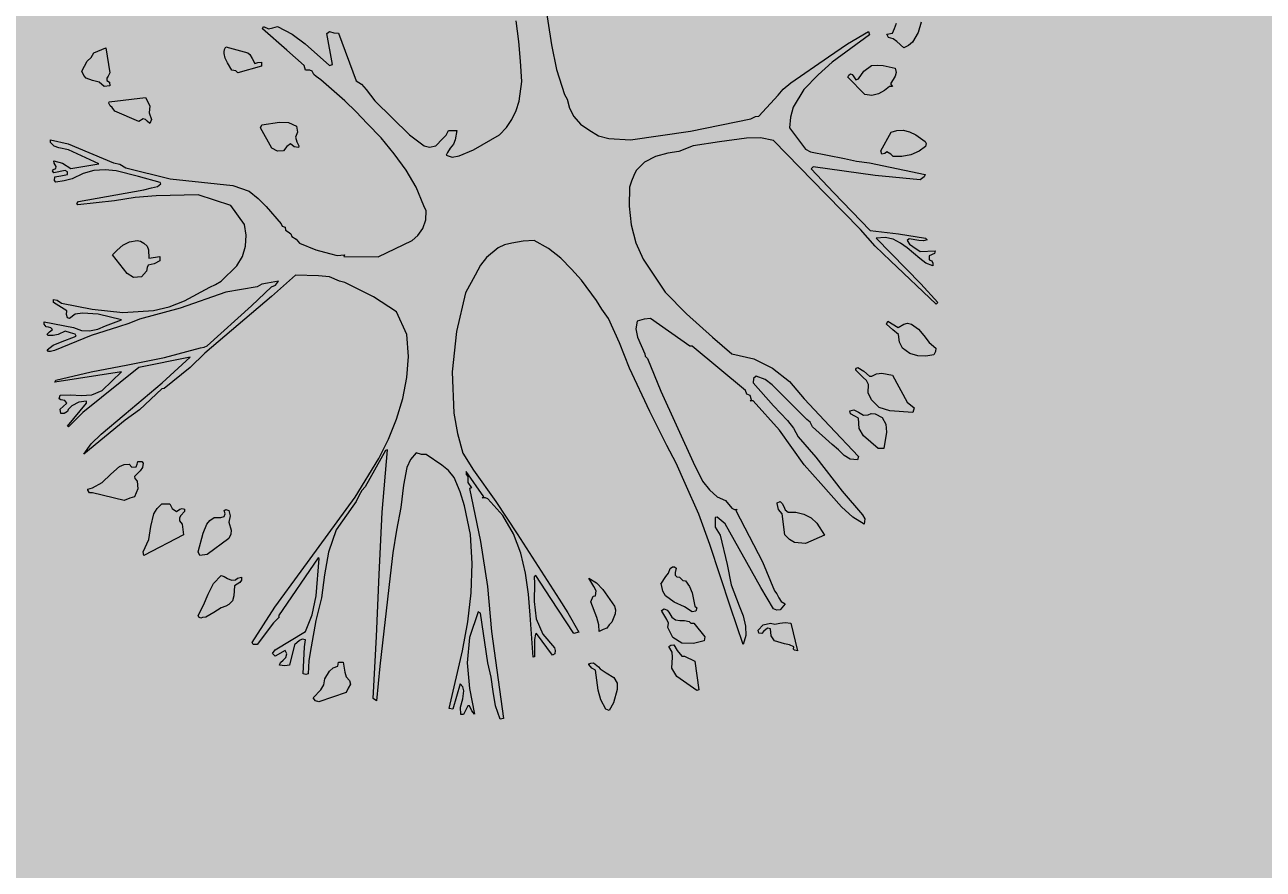
# Model space of a CAD drawing. Units: inches. Extents: x 84 to 1044, y -280 to 906.
# Tile 92 of 105: x 749 to 779, y 479 to 499. Entities that reach past the tile are written whole.
import ezdxf

# ---------------------------------------------------------------- set-up
doc = ezdxf.new("R2010")
doc.units = ezdxf.units.IN
doc.layers.add('A-ANNO-DIMS', color=2, linetype='Continuous', lineweight=18)
doc.layers.add('L-PLNT', color=114, linetype='Continuous', lineweight=15)
doc.layers.add('L-PLNT-PATT', color=9, linetype='Continuous', lineweight=9, true_color=0xafd9aa)
doc.styles.get("Standard").update_dxf_attribs({"font": 'arial.ttf'})
doc.dimstyles.get("Standard").update_dxf_attribs({"dimtxt": 0.18, "dimasz": 0.18, "dimexe": 0.18, "dimexo": 0.0625, "dimgap": 0.09, "dimtad": 0, "dimtih": 1, "dimtoh": 1, "dimdec": 4, "dimzin": 0, "dimdsep": 46, "dimtxsty": 'Standard', "dimcen": 0.09, "dimadec": 0, "dimazin": 0, "dimtfac": 1, "dimtdec": 4, "dimtofl": 0, "dimtmove": 0, "dimatfit": 3, "dimfxl": 1, "dimtolj": 1, "dimtzin": 0, "dimarcsym": 0})

# ---------------------------------------------------------------- blocks, each defined once
blk = doc.blocks.new('A$C37E508DF')
for p, q in [((0.7911, 1.1436), (0.8027, 1.0677)), ((0.7512, 1.0728), (0.7469, 1.1054)), ((1.3455, 1.0934), (1.3485, 1.102)), ((1.3875, 1.1037), (1.3828, 1.087)), ((0.3456, 1.093), (0.3469, 1.0964)), ((0.3842, 1.0591), (0.3456, 1.093)), ((0.3469, 1.0964), (0.355, 1.093)), ((0.355, 1.093), (0.3619, 1.0943)), ((0.3619, 1.0943), (0.3692, 1.0968)), ((0.3692, 1.0968), (0.3923, 1.0844)), ((0.3923, 1.0844), (0.4129, 1.069)), ((0.4472, 1.0857), (0.4515, 1.0887)), ((0.4562, 1.0364), (0.4472, 1.0857)), ((0.4515, 1.0887), (0.4584, 1.0865)), ((0.4584, 1.0865), (0.4657, 1.0861)), ((0.4657, 1.0861), (0.4939, 1.0107)), ((1.3057, 1.0835), (1.2469, 1.0402)), ((1.2713, 1.0694), (1.3044, 1.0887)), ((1.3044, 1.0887), (1.3057, 1.0835)), ((1.3335, 1.0844), (1.3421, 1.0861)), ((1.3361, 1.0793), (1.3335, 1.0844)), ((1.3434, 1.0771), (1.3361, 1.0793)), ((1.3421, 1.0861), (1.3455, 1.0934)), ((1.3828, 1.087), (1.3738, 1.072)), ((0.0789, 1.0552), (0.0978, 1.063)), ((0.0978, 1.063), (0.1042, 1.0231)), ((0.2847, 1.0565), (0.2856, 1.0604)), ((0.2856, 1.0604), (0.2877, 1.0647)), ((0.2877, 1.0647), (0.3224, 1.0552)), ((0.4112, 1.0351), (0.3842, 1.0591)), ((0.4129, 1.069), (0.4515, 1.0351)), ((0.7538, 1.0415), (0.7512, 1.0728)), ((0.8027, 1.0677), (0.8108, 1.0287)), ((1.2409, 1.0488), (1.2713, 1.0694)), ((1.349, 1.0728), (1.3434, 1.0771)), ((1.3605, 1.063), (1.349, 1.0728)), ((1.3678, 1.0664), (1.3605, 1.063)), ((1.3738, 1.072), (1.3678, 1.0664)), ((0.0596, 1.0257), (0.0682, 1.0415)), ((0.0682, 1.0415), (0.0746, 1.0475)), ((0.0746, 1.0475), (0.0789, 1.0552)), ((0.2851, 1.054), (0.2847, 1.0565)), ((0.2864, 1.0463), (0.2851, 1.054)), ((0.2899, 1.039), (0.2864, 1.0463)), ((0.2972, 1.0274), (0.2899, 1.039)), ((0.3224, 1.0552), (0.3255, 1.0522)), ((0.3255, 1.0522), (0.3293, 1.0458)), ((0.3293, 1.0458), (0.3336, 1.0381)), ((0.3336, 1.0381), (0.3383, 1.0398)), ((0.3383, 1.0398), (0.3439, 1.0402)), ((0.3439, 1.0402), (0.3439, 1.0338)), ((0.7559, 1.0098), (0.7538, 1.0415)), ((1.1813, 1.0072), (1.2409, 1.0488)), ((1.2469, 1.0402), (1.2246, 1.0201)), ((0.0626, 1.0188), (0.0596, 1.0257)), ((0.1042, 1.0231), (0.1012, 1.018)), ((0.3032, 1.0265), (0.2972, 1.0274)), ((0.3066, 1.0231), (0.3032, 1.0265)), ((0.3439, 1.0338), (0.3066, 1.0231)), ((0.4138, 1.0274), (0.4112, 1.0351)), ((0.4202, 1.0274), (0.4138, 1.0274)), ((0.4241, 1.0257), (0.4202, 1.0274)), ((0.4267, 1.0209), (0.4241, 1.0257)), ((0.4305, 1.0175), (0.4267, 1.0209)), ((0.4515, 1.0351), (0.4562, 1.0364)), ((0.8108, 1.0287), (0.8233, 0.9892)), ((1.2246, 1.0201), (1.2023, 0.9969)), ((1.2718, 1.0162), (1.2731, 1.0197)), ((1.2731, 1.0197), (1.2761, 1.0218)), ((1.2761, 1.0218), (1.2786, 1.0209)), ((1.2786, 1.0209), (1.2799, 1.0184)), ((1.2885, 1.0136), (1.2971, 1.0257)), ((1.2971, 1.0257), (1.3091, 1.0351)), ((1.3091, 1.0351), (1.3185, 1.0355)), ((1.3185, 1.0355), (1.3275, 1.0347)), ((1.3275, 1.0347), (1.3468, 1.0308)), ((1.3468, 1.0308), (1.3481, 1.0239)), ((1.3481, 1.0239), (1.3468, 1.018)), ((0.0665, 1.0149), (0.0626, 1.0188)), ((0.0763, 1.0111), (0.0665, 1.0149)), ((0.087, 1.0085), (0.0763, 1.0111)), ((0.0948, 1.0016), (0.087, 1.0085)), ((0.1042, 1.0029), (0.0948, 1.0016)), ((0.1012, 1.018), (0.099, 1.0149)), ((0.099, 1.0149), (0.099, 1.0111)), ((0.099, 1.0111), (0.1033, 1.0085)), ((0.1033, 1.0085), (0.1042, 1.0029)), ((0.4378, 1.0124), (0.4305, 1.0175)), ((0.476, 0.9789), (0.4378, 1.0124)), ((0.4939, 1.0107), (0.5021, 1.0051)), ((0.5021, 1.0051), (0.5094, 0.9969)), ((0.7516, 0.9785), (0.7559, 1.0098)), ((1.1693, 0.9974), (1.1813, 1.0072)), ((1.2984, 0.9892), (1.2718, 1.0162)), ((1.2799, 1.0184), (1.2842, 1.0124)), ((1.2842, 1.0124), (1.2885, 1.0136)), ((1.3378, 1.0016), (1.3297, 0.9952)), ((1.3421, 1.0016), (1.3378, 1.0016)), ((1.3468, 1.018), (1.3391, 1.0059)), ((1.3391, 1.0059), (1.3421, 1.0016)), ((0.1029, 0.9772), (0.1604, 0.9841)), ((0.1604, 0.9841), (0.1672, 0.9708)), ((0.5094, 0.9969), (0.5231, 0.9789)), ((0.8233, 0.9892), (0.8275, 0.9815)), ((0.8275, 0.9815), (0.8314, 0.9673)), ((1.1311, 0.9549), (1.1612, 0.9879)), ((1.1612, 0.9879), (1.1693, 0.9974)), ((1.2023, 0.9969), (1.1852, 0.9691)), ((1.3095, 0.9875), (1.2984, 0.9892)), ((1.3202, 0.9901), (1.3095, 0.9875)), ((1.3297, 0.9952), (1.3202, 0.9901)), ((0.1025, 0.9751), (0.1029, 0.9772)), ((0.1046, 0.9708), (0.1025, 0.9751)), ((0.1076, 0.9682), (0.1046, 0.9708)), ((0.1119, 0.9626), (0.1076, 0.9682)), ((0.1496, 0.9463), (0.1119, 0.9626)), ((0.1672, 0.9708), (0.1664, 0.9601)), ((0.4939, 0.9618), (0.476, 0.9789)), ((0.5111, 0.9429), (0.4939, 0.9618)), ((0.5231, 0.9789), (0.578, 0.9253)), ((0.7401, 0.9493), (0.7469, 0.9635)), ((0.7469, 0.9635), (0.7516, 0.9785)), ((0.8314, 0.9673), (0.8383, 0.954)), ((1.1852, 0.9691), (1.1809, 0.9532)), ((0.1565, 0.9506), (0.1496, 0.9463)), ((0.1604, 0.9493), (0.1565, 0.9506)), ((0.1629, 0.9468), (0.1604, 0.9493)), ((0.1672, 0.9429), (0.1629, 0.9468)), ((0.1664, 0.9601), (0.1698, 0.9493)), ((0.1698, 0.9493), (0.1672, 0.9429)), ((0.3426, 0.936), (0.3443, 0.9412)), ((0.3443, 0.9412), (0.3722, 0.9451)), ((0.3722, 0.9451), (0.3868, 0.9446)), ((0.3868, 0.9446), (0.3992, 0.9386)), ((0.5334, 0.9202), (0.5111, 0.9429)), ((0.7315, 0.9365), (0.7401, 0.9493)), ((0.8383, 0.954), (0.8486, 0.942)), ((0.8486, 0.942), (0.8619, 0.933)), ((1.0227, 0.9309), (1.1183, 0.9506)), ((1.1183, 0.9506), (1.1256, 0.954)), ((1.1256, 0.954), (1.1311, 0.9549)), ((1.1809, 0.9532), (1.1796, 0.936)), ((0.3602, 0.9039), (0.3426, 0.936)), ((0.4009, 0.9292), (0.3975, 0.9215)), ((0.3975, 0.9215), (0.3996, 0.9142)), ((0.3992, 0.9386), (0.4009, 0.9292)), ((0.578, 0.9253), (0.6011, 0.9077)), ((0.6303, 0.9189), (0.6359, 0.9245)), ((0.6359, 0.9245), (0.6397, 0.9322)), ((0.6397, 0.9322), (0.653, 0.9322)), ((0.653, 0.9322), (0.6505, 0.9172)), ((0.6796, 0.9013), (0.7203, 0.9253)), ((0.7203, 0.9253), (0.7315, 0.9365)), ((0.8619, 0.933), (0.8769, 0.9236)), ((0.8769, 0.9236), (0.8936, 0.9193)), ((0.9279, 0.9172), (1.0227, 0.9309)), ((1.1796, 0.936), (1.2049, 0.9022)), ((1.3241, 0.9), (1.3404, 0.9292)), ((1.3404, 0.9292), (1.3494, 0.9322)), ((1.3494, 0.9322), (1.3592, 0.9326)), ((1.3592, 0.9326), (1.3695, 0.93)), ((1.3695, 0.93), (1.3794, 0.9253)), ((1.3794, 0.9253), (1.394, 0.9146)), ((0.0103, 0.9129), (0.0103, 0.9172)), ((0.0103, 0.9172), (0.0382, 0.9107)), ((0.0159, 0.9073), (0.0103, 0.9129)), ((0.0232, 0.9043), (0.0159, 0.9073)), ((0.0386, 0.9013), (0.0232, 0.9043)), ((0.0382, 0.9107), (0.1098, 0.8807)), ((0.3692, 0.8992), (0.3602, 0.9039)), ((0.3838, 0.9069), (0.379, 0.9)), ((0.3898, 0.9107), (0.3838, 0.9069)), ((0.3958, 0.906), (0.3898, 0.9107)), ((0.4026, 0.9052), (0.3958, 0.906)), ((0.3996, 0.9142), (0.4031, 0.9077)), ((0.4031, 0.9077), (0.4026, 0.9052)), ((0.554, 0.8953), (0.5334, 0.9202)), ((0.6011, 0.9077), (0.6097, 0.9056)), ((0.6097, 0.9056), (0.6196, 0.9077)), ((0.6196, 0.9077), (0.6303, 0.9189)), ((0.6423, 0.9039), (0.6384, 0.8974)), ((0.6479, 0.9103), (0.6423, 0.9039)), ((0.6505, 0.9172), (0.6479, 0.9103)), ((0.8936, 0.9193), (0.9279, 0.9172)), ((1.0269, 0.9077), (1.0042, 0.8987)), ((1.0685, 0.9142), (1.0269, 0.9077)), ((1.1114, 0.9198), (1.0685, 0.9142)), ((1.1333, 0.9202), (1.1114, 0.9198)), ((1.1543, 0.9159), (1.1333, 0.9202)), ((1.2371, 0.8314), (1.1543, 0.9159)), ((1.2049, 0.9022), (1.2126, 0.8983)), ((1.3948, 0.9065), (1.3846, 0.8992)), ((1.394, 0.9146), (1.3957, 0.9112)), ((1.3957, 0.9112), (1.3948, 0.9065)), ((0.0159, 0.8803), (0.0154, 0.8837)), ((0.0154, 0.8837), (0.0292, 0.8803)), ((0.0866, 0.8794), (0.0386, 0.9013)), ((0.379, 0.9), (0.3692, 0.8992)), ((0.5728, 0.8691), (0.554, 0.8953)), ((0.6384, 0.8974), (0.6359, 0.8927)), ((0.6359, 0.8927), (0.6457, 0.8897)), ((0.6457, 0.8897), (0.6569, 0.8919)), ((0.6569, 0.8919), (0.6796, 0.9013)), ((0.9673, 0.8906), (0.9498, 0.8816)), ((0.9866, 0.8962), (0.9673, 0.8906)), ((1.0042, 0.8987), (0.9866, 0.8962)), ((1.2126, 0.8983), (1.2662, 0.8876)), ((1.2662, 0.8876), (1.2855, 0.8833)), ((1.2855, 0.8833), (1.3057, 0.8807)), ((1.3254, 0.8944), (1.3241, 0.9)), ((1.3301, 0.8957), (1.3254, 0.8944)), ((1.3335, 0.8983), (1.3301, 0.8957)), ((1.3395, 0.8944), (1.3335, 0.8983)), ((1.3434, 0.8906), (1.3395, 0.8944)), ((1.3571, 0.8906), (1.3434, 0.8906)), ((1.3713, 0.8936), (1.3571, 0.8906)), ((1.3846, 0.8992), (1.3713, 0.8936)), ((0.0133, 0.8679), (0.015, 0.87)), ((0.0154, 0.8649), (0.0133, 0.8679)), ((0.015, 0.87), (0.0184, 0.8717)), ((0.0334, 0.8687), (0.0154, 0.8649)), ((0.0176, 0.8777), (0.0159, 0.8803)), ((0.0193, 0.8752), (0.0176, 0.8777)), ((0.0184, 0.8717), (0.0193, 0.8752)), ((0.0266, 0.8602), (0.0369, 0.8623)), ((0.0292, 0.8803), (0.0424, 0.8717)), ((0.0369, 0.8666), (0.0334, 0.8687)), ((0.0369, 0.8623), (0.0369, 0.8666)), ((0.0424, 0.8717), (0.0866, 0.8794)), ((0.0617, 0.864), (0.0442, 0.8554)), ((0.0789, 0.8687), (0.0617, 0.864)), ((0.0965, 0.8696), (0.0789, 0.8687)), ((0.1141, 0.8679), (0.0965, 0.8696)), ((0.1098, 0.8807), (0.1196, 0.8786)), ((0.1492, 0.8593), (0.1141, 0.8679)), ((0.1196, 0.8786), (0.1295, 0.873)), ((0.1295, 0.873), (0.1994, 0.8554)), ((0.5887, 0.8421), (0.5728, 0.8691)), ((0.9369, 0.8687), (0.933, 0.861)), ((0.9498, 0.8816), (0.9369, 0.8687)), ((1.2169, 0.8743), (1.2135, 0.8713)), ((1.2135, 0.8713), (1.2491, 0.834)), ((1.3151, 0.8606), (1.2169, 0.8743)), ((1.3057, 0.8807), (1.394, 0.8623)), ((1.394, 0.8623), (1.3927, 0.8584)), ((0.0163, 0.8529), (0.0171, 0.8584)), ((0.0184, 0.8503), (0.0163, 0.8529)), ((0.0171, 0.8584), (0.0266, 0.8602)), ((0.0317, 0.8524), (0.0184, 0.8503)), ((0.0442, 0.8554), (0.0317, 0.8524)), ((0.1835, 0.8499), (0.1492, 0.8593)), ((0.1698, 0.8413), (0.1792, 0.8434)), ((0.1792, 0.8434), (0.1848, 0.8477)), ((0.1848, 0.8477), (0.1835, 0.8499)), ((0.1994, 0.8554), (0.2984, 0.8447)), ((0.2984, 0.8447), (0.3242, 0.8357)), ((0.9296, 0.852), (0.9262, 0.8421)), ((0.933, 0.861), (0.9296, 0.852)), ((1.3863, 0.8541), (1.3151, 0.8606)), ((1.3927, 0.8584), (1.3863, 0.8541)), ((0.0545, 0.8194), (0.1578, 0.8378)), ((0.1441, 0.8258), (0.1111, 0.8207)), ((0.1771, 0.8288), (0.1441, 0.8258)), ((0.1578, 0.8378), (0.1698, 0.8413)), ((0.2436, 0.8301), (0.1771, 0.8288)), ((0.2954, 0.813), (0.2436, 0.8301)), ((0.3242, 0.8357), (0.3387, 0.8241)), ((0.3387, 0.8241), (0.3512, 0.8117)), ((0.6007, 0.8125), (0.5887, 0.8421)), ((0.9262, 0.8421), (0.9257, 0.8121)), ((1.2919, 0.7752), (1.2371, 0.8314)), ((1.2491, 0.834), (1.3069, 0.7735)), ((0.0519, 0.8164), (0.0545, 0.8194)), ((0.0532, 0.8143), (0.0519, 0.8164)), ((0.1111, 0.8207), (0.0532, 0.8143)), ((0.3173, 0.7834), (0.2954, 0.813)), ((0.3512, 0.8117), (0.3748, 0.7842)), ((0.6046, 0.8048), (0.6007, 0.8125)), ((0.6037, 0.7903), (0.6046, 0.8048)), ((0.9257, 0.8121), (0.9287, 0.7825)), ((0.3748, 0.7842), (0.3765, 0.7804)), ((0.599, 0.777), (0.6037, 0.7903)), ((0.3199, 0.7662), (0.3173, 0.7834)), ((0.3186, 0.7491), (0.3199, 0.7662)), ((0.3765, 0.7804), (0.3816, 0.7791)), ((0.3816, 0.7791), (0.382, 0.7744)), ((0.382, 0.7744), (0.3859, 0.7714)), ((0.3859, 0.7714), (0.3902, 0.7684)), ((0.3902, 0.7684), (0.3919, 0.7641)), ((0.5823, 0.7577), (0.5913, 0.7658)), ((0.5913, 0.7658), (0.599, 0.777)), ((0.9287, 0.7825), (0.936, 0.7542)), ((1.3151, 0.7487), (1.2919, 0.7752)), ((1.3069, 0.7735), (1.352, 0.7684)), ((1.352, 0.7684), (1.3948, 0.7615)), ((0.1153, 0.7427), (0.1244, 0.7504)), ((0.1244, 0.7504), (0.1351, 0.7559)), ((0.1351, 0.7559), (0.1471, 0.7577)), ((0.1471, 0.7577), (0.1527, 0.7568)), ((0.1527, 0.7568), (0.1578, 0.7538)), ((0.1578, 0.7538), (0.1629, 0.7491)), ((0.1629, 0.7491), (0.1651, 0.7431)), ((0.3139, 0.7324), (0.3186, 0.7491)), ((0.3919, 0.7641), (0.3988, 0.7598)), ((0.3988, 0.7598), (0.4043, 0.7538)), ((0.4043, 0.7538), (0.4301, 0.7431)), ((0.5287, 0.7319), (0.5823, 0.7577)), ((0.7182, 0.7461), (0.7002, 0.7307)), ((0.7285, 0.7512), (0.7182, 0.7461)), ((0.7401, 0.7534), (0.7285, 0.7512)), ((0.7577, 0.7568), (0.7401, 0.7534)), ((0.7752, 0.7577), (0.7577, 0.7568)), ((0.798, 0.7452), (0.7752, 0.7577)), ((0.8173, 0.7298), (0.798, 0.7452)), ((0.936, 0.7542), (0.9476, 0.7285)), ((1.3391, 0.7255), (1.3151, 0.7487)), ((1.3309, 0.7624), (1.3164, 0.7615)), ((1.3164, 0.7615), (1.3871, 0.6891)), ((1.3434, 0.7598), (1.3309, 0.7624)), ((1.355, 0.7538), (1.3434, 0.7598)), ((1.3653, 0.7461), (1.355, 0.7538)), ((1.3854, 0.7294), (1.3653, 0.7461)), ((1.3687, 0.7607), (1.3657, 0.7577)), ((1.3657, 0.7577), (1.3691, 0.7521)), ((1.3841, 0.7577), (1.3687, 0.7607)), ((1.3691, 0.7521), (1.3743, 0.7482)), ((1.3743, 0.7482), (1.3863, 0.7405)), ((1.3914, 0.7572), (1.3841, 0.7577)), ((1.397, 0.759), (1.3914, 0.7572)), ((1.3948, 0.7615), (1.397, 0.759)), ((0.1081, 0.7349), (0.1153, 0.7427)), ((0.1312, 0.7058), (0.1081, 0.7349)), ((0.1651, 0.7431), (0.1655, 0.7298)), ((0.1655, 0.7298), (0.1831, 0.7324)), ((0.1831, 0.7255), (0.1741, 0.7208)), ((0.1831, 0.7324), (0.1831, 0.7255)), ((0.3049, 0.7178), (0.3139, 0.7324)), ((0.4301, 0.7431), (0.4515, 0.7371)), ((0.4515, 0.7371), (0.4635, 0.7341)), ((0.4635, 0.7341), (0.4755, 0.7349)), ((0.4755, 0.7349), (0.4742, 0.7324)), ((0.4742, 0.7324), (0.5287, 0.7319)), ((0.7002, 0.7307), (0.6903, 0.7186)), ((0.8344, 0.7122), (0.8173, 0.7298)), ((0.9476, 0.7285), (0.9828, 0.6762)), ((1.4116, 0.6569), (1.3391, 0.7255)), ((1.3953, 0.7221), (1.3854, 0.7294)), ((1.3863, 0.7405), (1.4099, 0.7414)), ((1.4086, 0.7375), (1.4004, 0.7337)), ((1.4004, 0.7337), (1.4004, 0.7272)), ((1.4004, 0.7272), (1.4047, 0.7255)), ((1.4047, 0.7255), (1.406, 0.7221)), ((1.4099, 0.7414), (1.4086, 0.7375)), ((0.1415, 0.6994), (0.1312, 0.7058)), ((0.1621, 0.7092), (0.1539, 0.7002)), ((0.1629, 0.7152), (0.1621, 0.7092)), ((0.1646, 0.7186), (0.1629, 0.7152)), ((0.1741, 0.7208), (0.1646, 0.7186)), ((0.28, 0.6933), (0.3049, 0.7178)), ((0.6903, 0.7186), (0.6818, 0.7032)), ((0.8503, 0.6951), (0.8344, 0.7122)), ((1.4064, 0.7178), (1.3953, 0.7221)), ((1.406, 0.7221), (1.4064, 0.7178)), ((0.1539, 0.7002), (0.1415, 0.6994)), ((0.262, 0.6839), (0.271, 0.6882)), ((0.271, 0.6882), (0.28, 0.6933)), ((0.3443, 0.6886), (0.337, 0.6843)), ((0.3533, 0.6903), (0.3443, 0.6886)), ((0.3709, 0.6933), (0.3533, 0.6903)), ((0.3975, 0.7028), (0.3598, 0.6693)), ((0.3598, 0.6843), (0.3662, 0.6873)), ((0.3662, 0.6873), (0.3709, 0.6933)), ((0.4339, 0.7019), (0.3975, 0.7028)), ((0.4515, 0.7002), (0.4339, 0.7019)), ((0.4674, 0.6933), (0.4515, 0.7002)), ((0.476, 0.6912), (0.4674, 0.6933)), ((0.4832, 0.6878), (0.476, 0.6912)), ((0.521, 0.6685), (0.4832, 0.6878)), ((0.6818, 0.7032), (0.6667, 0.6749)), ((0.8739, 0.6629), (0.8503, 0.6951)), ((1.3871, 0.6891), (1.4141, 0.6599)), ((0.2877, 0.6762), (0.2152, 0.6505)), ((0.2221, 0.6625), (0.262, 0.6839)), ((0.3598, 0.6693), (0.2543, 0.5797)), ((0.337, 0.6843), (0.2877, 0.6762)), ((0.328, 0.6543), (0.3598, 0.6843)), ((0.5578, 0.6449), (0.521, 0.6685)), ((0.6667, 0.6749), (0.6526, 0.614)), ((0.9828, 0.6762), (1.0162, 0.6415)), ((0.0146, 0.6599), (0.0146, 0.6642)), ((0.0146, 0.6642), (0.0206, 0.6633)), ((0.036, 0.6466), (0.0146, 0.6599)), ((0.0206, 0.6633), (0.0274, 0.6586)), ((0.0274, 0.6586), (0.0759, 0.6492)), ((0.0759, 0.6492), (0.1244, 0.644)), ((0.1244, 0.644), (0.1728, 0.647)), ((0.2152, 0.6505), (0.1509, 0.6333)), ((0.1728, 0.647), (0.1977, 0.6526)), ((0.1977, 0.6526), (0.2221, 0.6625)), ((0.2581, 0.5913), (0.328, 0.6543)), ((0.8824, 0.6492), (0.8739, 0.6629)), ((0.8932, 0.6342), (0.8824, 0.6492)), ((1.4141, 0.6599), (1.4116, 0.6569)), ((0, 0.629), (0.0467, 0.62)), ((0, 0.6252), (0, 0.629)), ((0.0356, 0.6406), (0.036, 0.6466)), ((0.0369, 0.6355), (0.0356, 0.6406)), ((0.0399, 0.6342), (0.0369, 0.6355)), ((0.0489, 0.641), (0.0399, 0.6342)), ((0.0609, 0.6428), (0.0489, 0.641)), ((0.0853, 0.641), (0.0609, 0.6428)), ((0.1226, 0.632), (0.0853, 0.641)), ((0.0973, 0.6226), (0.1226, 0.632)), ((0.1509, 0.6333), (0.1342, 0.6265)), ((0.5737, 0.6089), (0.5578, 0.6449)), ((0.9103, 0.5956), (0.8932, 0.6342)), ((0.9382, 0.6303), (0.936, 0.6179)), ((0.9493, 0.6333), (0.9382, 0.6303)), ((0.9596, 0.6342), (0.9493, 0.6333)), ((1.0218, 0.5904), (0.9596, 0.6342)), ((1.0162, 0.6415), (1.0574, 0.605)), ((1.3327, 0.6252), (1.3348, 0.6303)), ((1.3348, 0.6303), (1.3511, 0.62)), ((0.003, 0.6213), (0, 0.6252)), ((0.0069, 0.6204), (0.003, 0.6213)), ((0.0047, 0.6093), (0.0086, 0.6132)), ((0.0056, 0.6076), (0.0047, 0.6093)), ((0.0141, 0.6072), (0.0056, 0.6076)), ((0.0107, 0.6196), (0.0069, 0.6204)), ((0.0086, 0.6132), (0.0133, 0.617)), ((0.0133, 0.617), (0.0107, 0.6196)), ((0.0223, 0.6089), (0.0141, 0.6072)), ((0.0746, 0.6076), (0.0163, 0.5836)), ((0.0334, 0.6145), (0.0223, 0.6089)), ((0.0416, 0.6119), (0.0334, 0.6145)), ((0.0493, 0.6093), (0.0416, 0.6119)), ((0.0467, 0.62), (0.0592, 0.6153)), ((0.0506, 0.6063), (0.0493, 0.6093)), ((0.0592, 0.6153), (0.072, 0.6149)), ((0.072, 0.6149), (0.0849, 0.6175)), ((0.1175, 0.6213), (0.0746, 0.6076)), ((0.0849, 0.6175), (0.0973, 0.6226)), ((0.1342, 0.6265), (0.1175, 0.6213)), ((0.5763, 0.5741), (0.5737, 0.6089)), ((0.6526, 0.614), (0.6457, 0.5497)), ((0.936, 0.6179), (0.939, 0.605)), ((1.343, 0.6162), (1.3327, 0.6252)), ((1.352, 0.6089), (1.343, 0.6162)), ((1.3511, 0.62), (1.3601, 0.6256)), ((1.3533, 0.5969), (1.352, 0.6089)), ((1.3601, 0.6256), (1.3661, 0.6269)), ((1.3661, 0.6269), (1.3725, 0.6252)), ((1.3725, 0.6252), (1.3837, 0.6175)), ((1.3837, 0.6175), (1.3918, 0.6072)), ((0.0047, 0.5849), (0.0141, 0.5921)), ((0.0141, 0.5921), (0.0257, 0.5969)), ((0.0257, 0.5969), (0.0506, 0.6063)), ((0.2474, 0.5879), (0.253, 0.5892)), ((0.253, 0.5892), (0.2581, 0.5913)), ((0.9262, 0.5557), (0.9103, 0.5956)), ((0.939, 0.605), (0.9506, 0.5784)), ((1.0256, 0.5904), (1.0218, 0.5904)), ((1.1097, 0.5205), (1.0256, 0.5904)), ((1.0574, 0.605), (1.0883, 0.5784)), ((1.358, 0.5874), (1.3533, 0.5969)), ((1.3918, 0.6072), (1.4004, 0.5964)), ((1.4004, 0.5964), (1.4111, 0.5874)), ((0.0069, 0.5823), (0.0047, 0.5849)), ((0.0099, 0.5823), (0.0069, 0.5823)), ((0.0163, 0.5836), (0.0099, 0.5823)), ((0.1325, 0.5608), (0.1904, 0.5724)), ((0.2311, 0.5729), (0.1496, 0.557)), ((0.1869, 0.5325), (0.2311, 0.5729)), ((0.1904, 0.5724), (0.2474, 0.5879)), ((0.2543, 0.5797), (0.2311, 0.557)), ((0.5737, 0.5407), (0.5763, 0.5741)), ((0.9506, 0.5784), (0.951, 0.5746)), ((0.951, 0.5746), (0.9545, 0.5711)), ((0.9545, 0.5711), (0.9759, 0.5193)), ((1.0883, 0.5784), (1.123, 0.5703)), ((1.123, 0.5703), (1.1526, 0.5557)), ((1.37, 0.5789), (1.358, 0.5874)), ((1.3824, 0.575), (1.37, 0.5789)), ((1.3953, 0.5746), (1.3824, 0.575)), ((1.4077, 0.5771), (1.3953, 0.5746)), ((1.4103, 0.5823), (1.4077, 0.5771)), ((1.4111, 0.5874), (1.4103, 0.5823)), ((0.1226, 0.5497), (0.0171, 0.5338)), ((0.0184, 0.5368), (0.0746, 0.5501)), ((0.1496, 0.557), (0.0613, 0.4858)), ((0.0746, 0.5501), (0.1325, 0.5608)), ((0.0917, 0.5205), (0.1226, 0.5497)), ((0.2311, 0.557), (0.1899, 0.5235)), ((0.6457, 0.5497), (0.6483, 0.4845)), ((0.9583, 0.4871), (0.9262, 0.5557)), ((1.1526, 0.5557), (1.1792, 0.5347)), ((1.2842, 0.554), (1.2855, 0.5557)), ((1.2842, 0.5527), (1.2842, 0.554)), ((1.2958, 0.5407), (1.2842, 0.5527)), ((1.2855, 0.5557), (1.2876, 0.557)), ((1.2876, 0.557), (1.2971, 0.551)), ((1.2971, 0.551), (1.3057, 0.5433)), ((0.0171, 0.5338), (0.0184, 0.5368)), ((0.1269, 0.482), (0.1869, 0.5325)), ((0.5677, 0.5077), (0.5737, 0.5407)), ((1.1226, 0.5394), (1.1221, 0.5325)), ((1.1221, 0.5325), (1.1539, 0.4961)), ((1.1268, 0.5433), (1.1226, 0.5394)), ((1.141, 0.5377), (1.1268, 0.5433)), ((1.1521, 0.5296), (1.141, 0.5377)), ((1.1706, 0.5111), (1.1521, 0.5296)), ((1.1792, 0.5347), (1.2027, 0.5072)), ((1.3014, 0.536), (1.2958, 0.5407)), ((1.3044, 0.53), (1.3014, 0.536)), ((1.3039, 0.5167), (1.3044, 0.53)), ((1.3057, 0.5433), (1.3099, 0.5433)), ((1.3099, 0.5433), (1.3172, 0.5467)), ((1.3172, 0.5467), (1.3254, 0.548)), ((1.3254, 0.548), (1.3421, 0.5446)), ((1.3421, 0.5446), (1.3657, 0.5021)), ((0.024, 0.5072), (0.0253, 0.5128)), ((0.0253, 0.5128), (0.042, 0.5133)), ((0.042, 0.5133), (0.0587, 0.5124)), ((0.0587, 0.5124), (0.0755, 0.5133)), ((0.0755, 0.5133), (0.0917, 0.5205)), ((0.1861, 0.5231), (0.1509, 0.4897)), ((0.1899, 0.5235), (0.1861, 0.5231)), ((0.9759, 0.5193), (1.0269, 0.4069)), ((1.1118, 0.5145), (1.1097, 0.5205)), ((1.117, 0.5124), (1.1118, 0.5145)), ((1.1191, 0.5055), (1.117, 0.5124)), ((1.1955, 0.4858), (1.1706, 0.5111)), ((1.3091, 0.5055), (1.3039, 0.5167)), ((0.0262, 0.5055), (0.024, 0.5072)), ((0.0253, 0.491), (0.03, 0.4948)), ((0.0262, 0.4841), (0.0253, 0.491)), ((0.0326, 0.5047), (0.0262, 0.5055)), ((0.03, 0.4948), (0.036, 0.5004)), ((0.036, 0.5004), (0.0326, 0.5047)), ((0.0369, 0.4639), (0.0669, 0.5004)), ((0.0382, 0.4905), (0.0369, 0.4871)), ((0.0403, 0.4922), (0.0382, 0.4905)), ((0.0437, 0.4961), (0.0403, 0.4922)), ((0.0549, 0.5021), (0.0437, 0.4961)), ((0.0669, 0.5034), (0.0549, 0.5021)), ((0.0669, 0.5004), (0.0669, 0.5034)), ((0.5578, 0.4751), (0.5677, 0.5077)), ((1.117, 0.5042), (1.1191, 0.5055)), ((1.1217, 0.5042), (1.117, 0.5042)), ((1.1633, 0.4575), (1.1217, 0.5042)), ((1.1539, 0.4961), (1.1762, 0.4729)), ((1.2027, 0.5072), (1.2426, 0.4644)), ((1.3215, 0.4935), (1.3091, 0.5055)), ((1.3382, 0.4884), (1.3215, 0.4935)), ((1.3657, 0.5021), (1.3764, 0.4927)), ((1.3764, 0.4927), (1.3743, 0.4858)), ((0.0317, 0.4841), (0.0262, 0.4841)), ((0.0369, 0.4871), (0.0317, 0.4841)), ((0.0613, 0.4858), (0.0386, 0.4627)), ((0.1282, 0.4734), (0.0626, 0.4198)), ((0.0905, 0.4515), (0.1269, 0.482)), ((0.1509, 0.4897), (0.1282, 0.4734)), ((0.545, 0.4434), (0.5578, 0.4751)), ((0.6483, 0.4845), (0.6539, 0.4524)), ((0.9853, 0.4335), (0.9583, 0.4871)), ((1.1762, 0.4729), (1.1856, 0.4605)), ((1.207, 0.4747), (1.1955, 0.4858)), ((1.2122, 0.47), (1.207, 0.4747)), ((1.2748, 0.4884), (1.2812, 0.4897)), ((1.2761, 0.4832), (1.2748, 0.4884)), ((1.2825, 0.4798), (1.2761, 0.4832)), ((1.2812, 0.4897), (1.2885, 0.4862)), ((1.2885, 0.4764), (1.2825, 0.4798)), ((1.2885, 0.4862), (1.2962, 0.4815)), ((1.2894, 0.4601), (1.2885, 0.4764)), ((1.2962, 0.4815), (1.3039, 0.482)), ((1.3039, 0.482), (1.3087, 0.4841)), ((1.3087, 0.4841), (1.3147, 0.4832)), ((1.3147, 0.4832), (1.3258, 0.4777)), ((1.3258, 0.4777), (1.3318, 0.4669)), ((1.3743, 0.4858), (1.3382, 0.4884)), ((0.0386, 0.4627), (0.0369, 0.4639)), ((0.0746, 0.4361), (0.0905, 0.4515)), ((0.6539, 0.4524), (0.6625, 0.4211)), ((1.2027, 0.4026), (1.1633, 0.4575)), ((1.1856, 0.4605), (1.1933, 0.4468)), ((1.2156, 0.4627), (1.2122, 0.47)), ((1.2469, 0.4348), (1.2156, 0.4627)), ((1.2426, 0.4644), (1.2885, 0.4159)), ((1.2967, 0.4485), (1.2894, 0.4601)), ((1.3331, 0.4545), (1.3284, 0.4284)), ((1.3318, 0.4669), (1.3331, 0.4545)), ((0.0626, 0.4198), (0.0746, 0.4361)), ((0.5295, 0.4125), (0.545, 0.4434)), ((1.0003, 0.4052), (0.9853, 0.4335)), ((1.1933, 0.4468), (1.2212, 0.4146)), ((1.2568, 0.4266), (1.2469, 0.4348)), ((1.3082, 0.4386), (1.2967, 0.4485)), ((1.3198, 0.4284), (1.3082, 0.4386)), ((0.4922, 0.3516), (0.5295, 0.4125)), ((0.5403, 0.4254), (0.5081, 0.3679)), ((0.5347, 0.3276), (0.5433, 0.4266)), ((0.5433, 0.4266), (0.5403, 0.4254)), ((0.5887, 0.4215), (0.5797, 0.4112)), ((0.5969, 0.4189), (0.5887, 0.4215)), ((0.6046, 0.4189), (0.5969, 0.4189)), ((0.6295, 0.4022), (0.6046, 0.4189)), ((0.6625, 0.4211), (0.6796, 0.3945)), ((1.2212, 0.4146), (1.2628, 0.361)), ((1.2658, 0.4176), (1.2568, 0.4266)), ((1.2752, 0.4116), (1.2658, 0.4176)), ((1.2868, 0.4108), (1.2752, 0.4116)), ((1.2885, 0.4159), (1.2868, 0.4108)), ((1.3284, 0.4284), (1.3198, 0.4284)), ((0.1055, 0.388), (0.1192, 0.4001)), ((0.1192, 0.4001), (0.1265, 0.4031)), ((0.1265, 0.4031), (0.1346, 0.4039)), ((0.1346, 0.4039), (0.1389, 0.3992)), ((0.1389, 0.3992), (0.1458, 0.3996)), ((0.1518, 0.3932), (0.1432, 0.3842)), ((0.1458, 0.3996), (0.1471, 0.4035)), ((0.1471, 0.4035), (0.1484, 0.4082)), ((0.1484, 0.4082), (0.1548, 0.4082)), ((0.1556, 0.3983), (0.1518, 0.3932)), ((0.1548, 0.4082), (0.1565, 0.4052)), ((0.1565, 0.4052), (0.1556, 0.3983)), ((0.5741, 0.3983), (0.5686, 0.3705)), ((0.5797, 0.4112), (0.5741, 0.3983)), ((0.6397, 0.3936), (0.6295, 0.4022)), ((0.6487, 0.3825), (0.6397, 0.3936)), ((0.6796, 0.3945), (0.7148, 0.3447)), ((1.0145, 0.373), (1.0003, 0.4052)), ((1.0269, 0.4069), (1.0419, 0.3769)), ((1.2289, 0.373), (1.2027, 0.4026)), ((0.0763, 0.3662), (0.0917, 0.3748)), ((0.0917, 0.3748), (0.1055, 0.388)), ((0.1432, 0.3842), (0.1436, 0.3808)), ((0.1436, 0.3808), (0.1471, 0.3769)), ((0.1471, 0.3769), (0.1484, 0.3649)), ((0.6582, 0.3602), (0.6487, 0.3825)), ((0.6959, 0.352), (0.668, 0.3919)), ((0.668, 0.3919), (0.668, 0.3872)), ((0.668, 0.3872), (0.6706, 0.3842)), ((0.6706, 0.3842), (0.6702, 0.3748)), ((0.6702, 0.3748), (0.6762, 0.3662)), ((1.0359, 0.3246), (1.0145, 0.373)), ((1.0419, 0.3769), (1.0527, 0.3632)), ((1.2615, 0.3362), (1.2289, 0.373)), ((0.069, 0.364), (0.0763, 0.3662)), ((0.069, 0.3627), (0.069, 0.364)), ((0.0716, 0.3585), (0.069, 0.3627)), ((0.0763, 0.3585), (0.0716, 0.3585)), ((0.1269, 0.3464), (0.0763, 0.3585)), ((0.1484, 0.3649), (0.1432, 0.352)), ((0.4982, 0.3537), (0.4939, 0.3447)), ((0.5025, 0.3619), (0.4982, 0.3537)), ((0.5081, 0.3679), (0.5025, 0.3619)), ((0.5686, 0.3705), (0.5643, 0.3349)), ((0.665, 0.3379), (0.6582, 0.3602)), ((0.6762, 0.3662), (0.6732, 0.3653)), ((0.6732, 0.3653), (0.6903, 0.2813)), ((1.0527, 0.3632), (1.0647, 0.352)), ((1.2628, 0.361), (1.2949, 0.3233)), ((0.1355, 0.3499), (0.1269, 0.3464)), ((0.1432, 0.352), (0.1355, 0.3499)), ((0.1737, 0.325), (0.1788, 0.3336)), ((0.1788, 0.3336), (0.1861, 0.3409)), ((0.1861, 0.3409), (0.199, 0.3409)), ((0.199, 0.3409), (0.2024, 0.3336)), ((0.2024, 0.3336), (0.2097, 0.3289)), ((0.2148, 0.3323), (0.2182, 0.3336)), ((0.2182, 0.3336), (0.2221, 0.3327)), ((0.4065, 0.2345), (0.4922, 0.3516)), ((0.4884, 0.337), (0.4622, 0.2997)), ((0.4939, 0.3447), (0.4884, 0.337)), ((0.5643, 0.3349), (0.5578, 0.2993)), ((0.6745, 0.2924), (0.665, 0.3379)), ((0.6933, 0.3503), (0.6959, 0.352)), ((0.6985, 0.3503), (0.6933, 0.3503)), ((0.7023, 0.349), (0.6985, 0.3503)), ((0.7259, 0.3224), (0.7023, 0.349)), ((0.7148, 0.3447), (0.7487, 0.2937)), ((1.0647, 0.352), (1.078, 0.346)), ((1.078, 0.346), (1.0883, 0.334)), ((1.0883, 0.334), (1.0921, 0.3319)), ((1.1599, 0.3426), (1.1646, 0.3447)), ((1.1599, 0.3413), (1.1599, 0.3426)), ((1.162, 0.3319), (1.1599, 0.3413)), ((1.1646, 0.3447), (1.168, 0.3417)), ((1.168, 0.3417), (1.1702, 0.3366)), ((1.1702, 0.3366), (1.1727, 0.3314)), ((1.2795, 0.3199), (1.2615, 0.3362)), ((0.1689, 0.3053), (0.1737, 0.325)), ((0.2097, 0.3289), (0.2148, 0.3323)), ((0.2161, 0.3224), (0.214, 0.3186)), ((0.214, 0.3186), (0.214, 0.3139)), ((0.214, 0.3139), (0.2182, 0.3087)), ((0.2221, 0.3289), (0.2161, 0.3224)), ((0.2221, 0.3327), (0.2221, 0.3289)), ((0.2577, 0.3087), (0.2624, 0.3147)), ((0.2624, 0.3147), (0.2689, 0.3194)), ((0.2689, 0.3194), (0.2796, 0.3194)), ((0.2796, 0.3194), (0.2847, 0.3211)), ((0.2847, 0.3211), (0.2864, 0.325)), ((0.2851, 0.3302), (0.2877, 0.3319)), ((0.2864, 0.325), (0.2851, 0.3302)), ((0.2877, 0.3319), (0.292, 0.3306)), ((0.292, 0.3306), (0.2941, 0.322)), ((0.2941, 0.322), (0.292, 0.3117)), ((0.53, 0.229), (0.5347, 0.3276)), ((0.7427, 0.2937), (0.7259, 0.3224)), ((1.0535, 0.2766), (1.0359, 0.3246)), ((1.0647, 0.3199), (1.0617, 0.3194)), ((1.0617, 0.3194), (1.0617, 0.304)), ((1.0711, 0.3147), (1.0647, 0.3199)), ((1.0775, 0.3092), (1.0711, 0.3147)), ((1.0921, 0.3319), (1.0968, 0.3319)), ((1.0968, 0.3319), (1.0947, 0.3306)), ((1.0947, 0.3306), (1.1367, 0.2491)), ((1.1676, 0.325), (1.162, 0.3319)), ((1.1719, 0.292), (1.1676, 0.325)), ((1.1727, 0.3314), (1.177, 0.3276)), ((1.177, 0.3276), (1.1895, 0.3276)), ((1.1895, 0.3276), (1.2019, 0.3246)), ((1.2019, 0.3246), (1.2135, 0.3186)), ((1.2135, 0.3186), (1.2225, 0.3104)), ((1.2975, 0.3087), (1.2795, 0.3199)), ((1.2949, 0.3233), (1.2988, 0.3173)), ((1.2988, 0.3173), (1.2975, 0.3087)), ((0.1655, 0.2843), (0.1689, 0.3053)), ((0.2182, 0.3087), (0.2204, 0.292)), ((0.2436, 0.265), (0.2517, 0.2946)), ((0.2517, 0.2946), (0.2577, 0.3087)), ((0.292, 0.3117), (0.2959, 0.2993)), ((0.2959, 0.2993), (0.2954, 0.2928)), ((0.4622, 0.2997), (0.4502, 0.2645)), ((0.5578, 0.2993), (0.5518, 0.2633)), ((1.0617, 0.304), (1.0698, 0.2911)), ((1.1341, 0.2084), (1.0775, 0.3092)), ((1.2225, 0.3104), (1.2349, 0.2911)), ((0.1565, 0.265), (0.1655, 0.2843)), ((0.2204, 0.292), (0.1578, 0.259)), ((0.292, 0.286), (0.2581, 0.2607)), ((0.2954, 0.2928), (0.292, 0.286)), ((0.6775, 0.2465), (0.6745, 0.2924)), ((0.6903, 0.2813), (0.7015, 0.2101)), ((0.7542, 0.2628), (0.7427, 0.2937)), ((0.7487, 0.2937), (0.8151, 0.1899)), ((1.0861, 0.1775), (1.0535, 0.2766)), ((1.0698, 0.2911), (1.0805, 0.2448)), ((1.1792, 0.2847), (1.1719, 0.292)), ((1.1873, 0.28), (1.1792, 0.2847)), ((1.2049, 0.2783), (1.1873, 0.28)), ((1.2349, 0.2911), (1.2049, 0.2783)), ((0.1578, 0.259), (0.1565, 0.265)), ((0.2461, 0.259), (0.2436, 0.265)), ((0.2581, 0.2607), (0.2461, 0.259)), ((0.4335, 0.2556), (0.3709, 0.1634)), ((0.4352, 0.2543), (0.4335, 0.2556)), ((0.4502, 0.2645), (0.4438, 0.2285)), ((0.5518, 0.2633), (0.5475, 0.2268)), ((0.7615, 0.2311), (0.7542, 0.2628)), ((0.4305, 0.1951), (0.4352, 0.2543)), ((0.6758, 0.2002), (0.6775, 0.2465)), ((0.9879, 0.2311), (0.9905, 0.2384)), ((0.9905, 0.2384), (0.9943, 0.241)), ((0.9943, 0.241), (0.9973, 0.2414)), ((0.9973, 0.2414), (1.0003, 0.2393)), ((1.0003, 0.2393), (0.9986, 0.232)), ((1.0805, 0.2448), (1.087, 0.2127)), ((1.1367, 0.2491), (1.1556, 0.2032)), ((0.268, 0.2148), (0.28, 0.2277)), ((0.28, 0.2277), (0.2851, 0.226)), ((0.2851, 0.226), (0.2903, 0.2225)), ((0.2903, 0.2225), (0.2963, 0.22)), ((0.2963, 0.22), (0.3027, 0.2204)), ((0.3096, 0.2165), (0.301, 0.211)), ((0.3027, 0.2204), (0.3061, 0.2234)), ((0.3061, 0.2234), (0.3122, 0.2247)), ((0.3122, 0.22), (0.3096, 0.2165)), ((0.3122, 0.2247), (0.3122, 0.22)), ((0.3649, 0.1775), (0.4065, 0.2345)), ((0.4438, 0.2285), (0.4391, 0.1921)), ((0.5261, 0.1308), (0.53, 0.229)), ((0.5475, 0.2268), (0.5313, 0.084)), ((0.7662, 0.1981), (0.7615, 0.2311)), ((0.7778, 0.2277), (0.7752, 0.2255)), ((0.7752, 0.2255), (0.7761, 0.2152)), ((0.8018, 0.1912), (0.7778, 0.2277)), ((0.8619, 0.2234), (0.8739, 0.2161)), ((0.87, 0.2101), (0.8619, 0.2234)), ((0.8739, 0.2161), (0.8841, 0.2054)), ((0.9759, 0.214), (0.9836, 0.226)), ((0.9836, 0.226), (0.9879, 0.2311)), ((0.9986, 0.232), (0.9986, 0.2281)), ((0.9986, 0.2281), (1.0012, 0.2255)), ((1.0012, 0.2255), (1.0051, 0.2251)), ((1.0051, 0.2251), (1.0076, 0.2225)), ((1.0076, 0.2225), (1.0106, 0.2195)), ((1.0106, 0.2195), (1.0149, 0.2191)), ((1.0149, 0.2191), (1.0214, 0.2101)), ((0.2521, 0.1805), (0.2594, 0.1981)), ((0.2594, 0.1981), (0.268, 0.2148)), ((0.301, 0.211), (0.3002, 0.1951)), ((0.6706, 0.1539), (0.6758, 0.2002)), ((0.7015, 0.2101), (0.7079, 0.1389)), ((0.7688, 0.1646), (0.7662, 0.1981)), ((0.7761, 0.2152), (0.7752, 0.1861)), ((0.8734, 0.2032), (0.87, 0.2101)), ((0.8726, 0.1955), (0.8734, 0.2032)), ((0.8841, 0.2054), (0.9026, 0.1792)), ((0.9768, 0.2127), (0.9759, 0.214)), ((0.9789, 0.2028), (0.9768, 0.2127)), ((0.9832, 0.1955), (0.9789, 0.2028)), ((1.0214, 0.2101), (1.0252, 0.2002)), ((1.0252, 0.2002), (1.0295, 0.1788)), ((1.087, 0.2127), (1.0998, 0.1797)), ((1.1543, 0.1749), (1.1341, 0.2084)), ((1.1556, 0.2032), (1.1594, 0.1985)), ((1.1594, 0.1985), (1.1624, 0.1921)), ((0.2436, 0.1642), (0.2521, 0.1805)), ((0.2873, 0.1788), (0.28, 0.1762)), ((0.292, 0.1818), (0.2873, 0.1788)), ((0.298, 0.1874), (0.292, 0.1818)), ((0.3002, 0.1951), (0.298, 0.1874)), ((0.3293, 0.1213), (0.3649, 0.1775)), ((0.4241, 0.1651), (0.4305, 0.1951)), ((0.4391, 0.1921), (0.4301, 0.1561)), ((0.7752, 0.1861), (0.7787, 0.1591)), ((0.8383, 0.1359), (0.8018, 0.1912)), ((0.8151, 0.1899), (0.8288, 0.1685)), ((0.8649, 0.1857), (0.8687, 0.1947)), ((0.8743, 0.1608), (0.8649, 0.1857)), ((0.8687, 0.1947), (0.8726, 0.1955)), ((0.9026, 0.1792), (0.9043, 0.1732)), ((0.9969, 0.1852), (0.9832, 0.1955)), ((1.0132, 0.1779), (0.9969, 0.1852)), ((1.0256, 0.1698), (1.0132, 0.1779)), ((1.0295, 0.1788), (1.0325, 0.1762)), ((1.1063, 0.1183), (1.0861, 0.1775)), ((1.0998, 0.1797), (1.1058, 0.1634)), ((1.1624, 0.1921), (1.1663, 0.1861)), ((1.1727, 0.1827), (1.1646, 0.1732)), ((1.1663, 0.1861), (1.1727, 0.1827)), ((0.2448, 0.1616), (0.2436, 0.1642)), ((0.2478, 0.1599), (0.2448, 0.1616)), ((0.2508, 0.1608), (0.2478, 0.1599)), ((0.2556, 0.1616), (0.2508, 0.1608)), ((0.2684, 0.1689), (0.2556, 0.1616)), ((0.28, 0.1762), (0.2684, 0.1689)), ((0.3692, 0.1591), (0.3628, 0.1526)), ((0.3718, 0.1616), (0.3692, 0.1591)), ((0.3709, 0.1634), (0.3718, 0.1616)), ((0.4138, 0.1389), (0.4241, 0.1651)), ((0.6865, 0.1698), (0.6732, 0.1295)), ((0.6903, 0.1681), (0.6865, 0.1698)), ((0.7023, 0.0892), (0.6903, 0.1681)), ((0.774, 0.0982), (0.7688, 0.1646)), ((0.7787, 0.1591), (0.789, 0.1346)), ((0.8288, 0.1685), (0.846, 0.1376)), ((0.8777, 0.1496), (0.8743, 0.1608)), ((0.9035, 0.1668), (0.8983, 0.1535)), ((0.9043, 0.1732), (0.9035, 0.1668)), ((0.9768, 0.1719), (0.9811, 0.1749)), ((0.9776, 0.1711), (0.9768, 0.1719)), ((0.9853, 0.1578), (0.9776, 0.1711)), ((0.9811, 0.1749), (0.9858, 0.1728)), ((0.9879, 0.1518), (0.9853, 0.1578)), ((0.9858, 0.1728), (0.9884, 0.1694)), ((0.9884, 0.1694), (0.9931, 0.1616)), ((0.9931, 0.1616), (0.9991, 0.1574)), ((0.9991, 0.1574), (1.0059, 0.1565)), ((1.0312, 0.1711), (1.0256, 0.1698)), ((1.0325, 0.1762), (1.0312, 0.1711)), ((1.1058, 0.1634), (1.1097, 0.1475)), ((1.1594, 0.1728), (1.1543, 0.1749)), ((1.1646, 0.1732), (1.1594, 0.1728)), ((0.3628, 0.1526), (0.337, 0.1183)), ((0.3653, 0.1098), (0.4138, 0.1389)), ((0.4301, 0.1561), (0.4224, 0.1145)), ((0.662, 0.108), (0.6706, 0.1539)), ((0.7079, 0.1389), (0.7268, 0.0013)), ((0.846, 0.1376), (0.8383, 0.1359)), ((0.8781, 0.1389), (0.8777, 0.1496)), ((0.8846, 0.1419), (0.8781, 0.1389)), ((0.8902, 0.1441), (0.8846, 0.1419)), ((0.894, 0.1496), (0.8902, 0.1441)), ((0.8983, 0.1535), (0.894, 0.1496)), ((0.9866, 0.1453), (0.9879, 0.1518)), ((0.9948, 0.1291), (0.9866, 0.1453)), ((1.0059, 0.1565), (1.0132, 0.1565)), ((1.0132, 0.1565), (1.0205, 0.1548)), ((1.0205, 0.1548), (1.0235, 0.1522)), ((1.0235, 0.1522), (1.0282, 0.1518)), ((1.0282, 0.1518), (1.0454, 0.1303)), ((1.1097, 0.1475), (1.1101, 0.1325)), ((1.1298, 0.1411), (1.1376, 0.1492)), ((1.1311, 0.1364), (1.1298, 0.1411)), ((1.1384, 0.1389), (1.1354, 0.1359)), ((1.1376, 0.1492), (1.1491, 0.1518)), ((1.1423, 0.1423), (1.1384, 0.1389)), ((1.1449, 0.1441), (1.1423, 0.1423)), ((1.1491, 0.1428), (1.1449, 0.1441)), ((1.1491, 0.1518), (1.1564, 0.1505)), ((1.1504, 0.132), (1.1491, 0.1428)), ((1.1564, 0.1505), (1.1642, 0.1518)), ((1.1642, 0.1518), (1.1727, 0.1531)), ((1.1727, 0.1531), (1.1813, 0.1518)), ((1.1813, 0.1518), (1.192, 0.108)), ((0.3306, 0.1183), (0.3293, 0.1213)), ((0.337, 0.1183), (0.3306, 0.1183)), ((0.4039, 0.1248), (0.3962, 0.1175)), ((0.4082, 0.1269), (0.4039, 0.1248)), ((0.4134, 0.1256), (0.4082, 0.1269)), ((0.4121, 0.1145), (0.4134, 0.1256)), ((0.5205, 0.033), (0.5261, 0.1308)), ((0.6732, 0.1295), (0.6693, 0.0892)), ((0.7774, 0.1346), (0.7757, 0.1261)), ((0.7757, 0.1261), (0.7761, 0.117)), ((0.7791, 0.1359), (0.7774, 0.1346)), ((0.8044, 0.1012), (0.7791, 0.1359)), ((0.789, 0.1346), (0.8074, 0.1132)), ((1.0089, 0.1205), (0.9948, 0.1291)), ((1.0274, 0.12), (1.0089, 0.1205)), ((1.0441, 0.1239), (1.0274, 0.12)), ((1.0454, 0.1303), (1.0441, 0.1239)), ((1.1101, 0.1325), (1.1063, 0.1183)), ((1.1354, 0.1359), (1.1311, 0.1364)), ((1.1556, 0.1239), (1.1504, 0.132)), ((1.1714, 0.1192), (1.1556, 0.1239)), ((1.1792, 0.1179), (1.1714, 0.1192)), ((1.186, 0.1145), (1.1792, 0.1179)), ((0.3615, 0.1042), (0.3653, 0.1098)), ((0.3653, 0.0999), (0.3615, 0.1042)), ((0.3812, 0.1089), (0.3653, 0.0999)), ((0.3842, 0.1037), (0.3812, 0.1089)), ((0.3825, 0.0978), (0.3842, 0.1037)), ((0.3962, 0.1175), (0.3885, 0.0853)), ((0.4099, 0.0716), (0.4121, 0.1145)), ((0.4224, 0.1145), (0.4189, 0.093)), ((0.641, 0.0172), (0.662, 0.108)), ((0.7761, 0.099), (0.774, 0.0982)), ((0.7761, 0.117), (0.7761, 0.099)), ((0.8083, 0.1037), (0.8044, 0.1012)), ((0.8074, 0.1132), (0.8087, 0.1089)), ((0.8087, 0.1089), (0.8083, 0.1037)), ((0.9884, 0.1149), (0.9918, 0.117)), ((0.9935, 0.1063), (0.9884, 0.1149)), ((0.9918, 0.117), (0.9961, 0.1175)), ((0.9931, 0.081), (0.9943, 0.0982)), ((0.9943, 0.0982), (0.9935, 0.1063)), ((0.9961, 0.1175), (1.0016, 0.1085)), ((1.0016, 0.1085), (1.0089, 0.0999)), ((1.0089, 0.0999), (1.0132, 0.0999)), ((1.0132, 0.0999), (1.0295, 0.0917)), ((1.1856, 0.111), (1.186, 0.1145)), ((1.1873, 0.1093), (1.1856, 0.111)), ((1.192, 0.108), (1.1873, 0.1093)), ((0.3722, 0.0853), (0.3739, 0.09)), ((0.3808, 0.0845), (0.3722, 0.0853)), ((0.3739, 0.09), (0.3782, 0.0935)), ((0.3782, 0.0935), (0.3825, 0.0978)), ((0.3885, 0.0853), (0.3808, 0.0845)), ((0.4189, 0.093), (0.4176, 0.072)), ((0.4515, 0.0763), (0.4571, 0.0815)), ((0.4571, 0.0815), (0.4648, 0.084)), ((0.4648, 0.084), (0.4657, 0.0905)), ((0.4657, 0.0905), (0.473, 0.0905)), ((0.473, 0.0905), (0.476, 0.0746)), ((0.5313, 0.084), (0.5257, 0.0291)), ((0.6693, 0.0892), (0.6728, 0.0484)), ((0.7075, 0.0665), (0.7023, 0.0892)), ((0.8619, 0.0875), (0.8649, 0.0887)), ((0.8619, 0.0866), (0.8619, 0.0875)), ((0.8666, 0.0806), (0.8619, 0.0866)), ((0.8649, 0.0887), (0.8691, 0.0892)), ((0.8726, 0.0776), (0.8666, 0.0806)), ((0.8691, 0.0892), (0.8769, 0.0827)), ((0.8769, 0.0827), (0.8799, 0.0797)), ((0.8799, 0.0797), (0.8893, 0.0733)), ((1.0012, 0.0677), (0.9931, 0.081)), ((1.0295, 0.0917), (1.0359, 0.0463)), ((0.4142, 0.0707), (0.4099, 0.0716)), ((0.4176, 0.072), (0.4142, 0.0707)), ((0.4425, 0.0544), (0.4442, 0.0639)), ((0.4442, 0.0639), (0.4515, 0.0763)), ((0.476, 0.0746), (0.4777, 0.0673)), ((0.4777, 0.0673), (0.4832, 0.0613)), ((0.4832, 0.0613), (0.4845, 0.0553)), ((0.7105, 0.0437), (0.7075, 0.0665)), ((0.8764, 0.0459), (0.8726, 0.0776)), ((0.8893, 0.0733), (0.9013, 0.066)), ((0.9013, 0.066), (0.9069, 0.057)), ((1.0325, 0.0454), (1.0012, 0.0677)), ((0.4258, 0.0339), (0.4378, 0.0463)), ((0.4777, 0.0424), (0.4348, 0.0274)), ((0.4378, 0.0463), (0.4425, 0.0544)), ((0.4811, 0.0493), (0.4777, 0.0424)), ((0.4845, 0.0553), (0.4811, 0.0493)), ((0.6582, 0.0562), (0.6466, 0.0159)), ((0.6625, 0.051), (0.6582, 0.0562)), ((0.6642, 0.045), (0.6625, 0.051)), ((0.6625, 0.0321), (0.6642, 0.045)), ((0.6728, 0.0484), (0.6809, 0.0082)), ((0.7144, 0.0214), (0.7105, 0.0437)), ((0.8807, 0.0304), (0.8764, 0.0459)), ((0.9069, 0.0471), (0.9009, 0.0261)), ((0.9069, 0.057), (0.9069, 0.0471)), ((1.0359, 0.0463), (1.0325, 0.0454)), ((0.4296, 0.0291), (0.4258, 0.0339)), ((0.4348, 0.0274), (0.4296, 0.0291)), ((0.5257, 0.0291), (0.5205, 0.033)), ((0.659, 0.0193), (0.6625, 0.0321)), ((0.6702, 0.0214), (0.6637, 0.0077)), ((0.6732, 0.0214), (0.6702, 0.0214)), ((0.6766, 0.0133), (0.6732, 0.0214)), ((0.7216, 0), (0.7144, 0.0214)), ((0.8889, 0.0159), (0.8807, 0.0304)), ((0.9009, 0.0261), (0.894, 0.0137)), ((0.6466, 0.0159), (0.641, 0.0172)), ((0.6595, 0.0077), (0.659, 0.0193)), ((0.6637, 0.0077), (0.6595, 0.0077)), ((0.6809, 0.0082), (0.6766, 0.0133)), ((0.7268, 0.0013), (0.7216, 0)), ((0.894, 0.0137), (0.8889, 0.0159))]:
    blk.add_line(p, q)
blk = doc.blocks.new('*D62')
at = {"layer": 'A-ANNO-DIMS', "color": 0, "lineweight": -2, "transparency": 16777216}
for p, q in [((203.179, 709.183), (203.179, 905.9)), ((896.074, 400.183), (896.074, 905.9)), ((203.359, 905.72), (549.232, 905.72)), ((895.894, 905.72), (550.021, 905.72))]:
    blk.add_line(p, q, dxfattribs=at)
at = {"layer": 'A-ANNO-DIMS', "color": 0, "transparency": 16777216}
for points in [[(203.359, 905.75), (203.359, 905.69), (203.179, 905.72)], [(895.894, 905.75), (895.894, 905.69), (896.074, 905.72)]]:
    blk.add_solid(points, dxfattribs=at)
at = {"layer": 'Defpoints', "color": 0, "transparency": 16777216}
for p in [(896.074, 905.72), (203.179, 709.12), (896.074, 400.12)]:
    blk.add_point(p, dxfattribs=at)
at = {"layer": 'A-ANNO-DIMS', "color": 0, "transparency": 16777216, "insert": (549.627, 905.72), "char_height": 0.18, "attachment_point": 5}
blk.add_mtext('\\A1;692.9', dxfattribs=at)

msp = doc.modelspace()

# ---------------------------------------------------------------- hatches: boundary and pattern name
at = {"layer": 'L-PLNT-PATT', "transparency": 33554597}
h = msp.add_hatch(color=256, dxfattribs=at)
h.dxf.hatch_style = 1
h.paths.add_polyline_path([(896.074, 511.12), (704.074, 511.12), (704.074, 491.62), (704.074, 419.62), (704.074, 400.12), (833.074, 400.12), (896.074, 400.12)])

# ---------------------------------------------------------------- block references
at = {"layer": 'L-PLNT', "xscale": 15.19586232982809, "yscale": 15.19586232982809, "zscale": 15.19586232982809}
msp.add_blockref('A$C37E508DF', (749.806, 482.553), dxfattribs=at)

# ---------------------------------------------------------------- dimensions: what is measured, and where the dimension line sits
at = {"layer": 'A-ANNO-DIMS'}
dim = msp.add_linear_dim(base=(896.074, 905.72), p1=(203.179, 709.12), p2=(896.074, 400.12), dimstyle='Standard', override={"dimdec": 1, "dimlfac": 1, "dimrnd": 0, "dimzin": 0, "dimdsep": 46, "dimlunit": 2}, dxfattribs=at)
dim.commit()
dim.dimension.update_dxf_attribs({"geometry": '*D62', "text_midpoint": (549.627, 905.72)})

doc.saveas('drawing.dxf')
